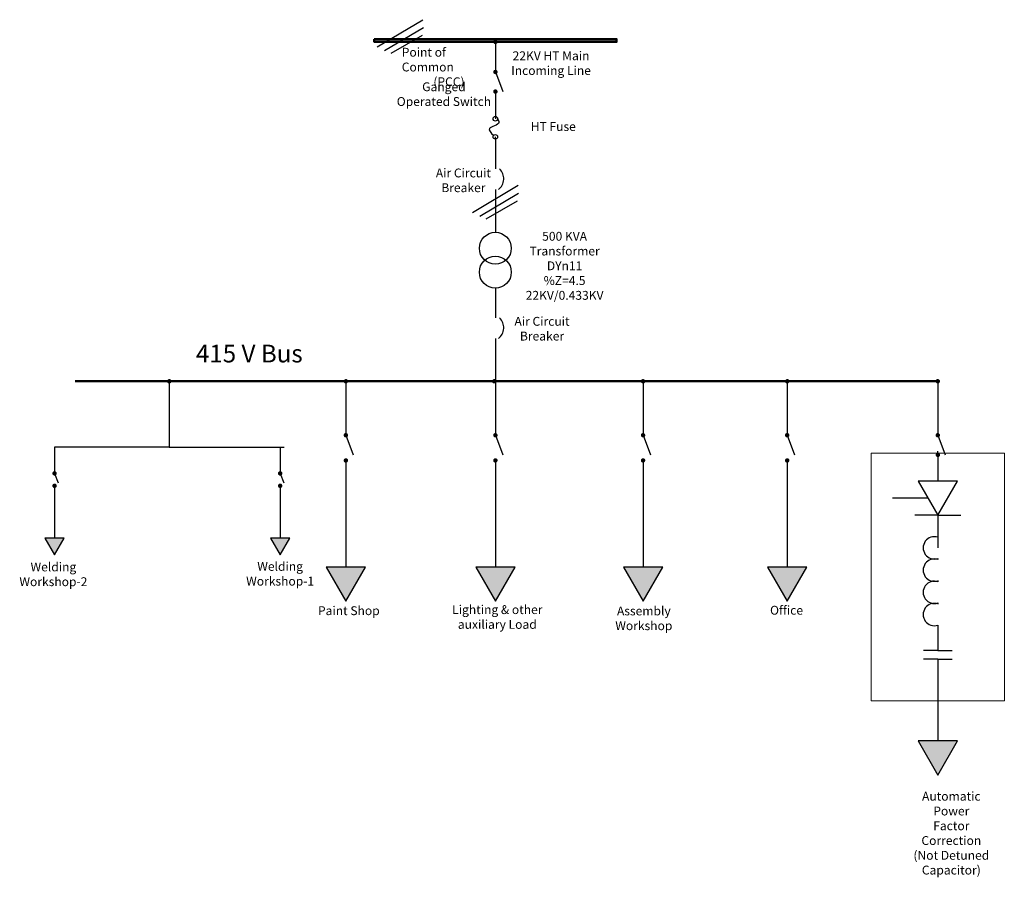
# Model space of a CAD drawing. Units: millimetres. Extents: x 147 to 258, y 68 to 165.
import ezdxf

# ---------------------------------------------------------------- set-up
doc = ezdxf.new("R2010")
doc.units = ezdxf.units.MM
doc.header["$MEASUREMENT"] = 0
for name, color, linetype, lineweight in [('E-ANNO-TEXT', 3, 'Continuous', 18), ('E-EQPM-BNDY', 8, 'Continuous', 18), ('E-POWR-BUSW', 1, 'Continuous', 50), ('E-POWR-WIRE', 7, 'Continuous', 25), ('E-SYMB', 4, 'Continuous', 25)]:
    doc.layers.add(name, color=color, linetype=linetype, lineweight=lineweight)
doc.styles.get("Standard").update_dxf_attribs({"font": 'arial.ttf'})

# ---------------------------------------------------------------- blocks, each defined once
blk = doc.blocks.new('LOAD-SYMBOL')
h = blk.add_hatch(color=256)
h.dxf.hatch_style = 1
h.paths.add_polyline_path([(202.61, 103), (198.16, 103), (200.38, 99.15)])
blk.add_lwpolyline([(200.38, 99.15), (202.61, 103), (198.16, 103)], close=True)
blk = doc.blocks.new('LOAD-SYMBOL-SMALL')
h = blk.add_hatch(color=256)
h.dxf.hatch_style = 1
h.paths.add_polyline_path([(150.59, 104.4), (151.68, 106.29), (149.5, 106.29)])
blk.add_lwpolyline([(150.59, 104.4), (151.68, 106.29), (149.5, 106.29)], close=True)
blk = doc.blocks.new('SWITCH-ISOLATOR')
blk.add_line((200.38, 117.9), (201.22, 115.7))
at = {"const_width": 0.25}
for points in [[(200.26, 117.9, 1), (200.51, 117.9, 1)], [(200.26, 115.05, 1), (200.51, 115.05, 1)]]:
    blk.add_lwpolyline(points, format="xyb", close=True, dxfattribs=at)
blk = doc.blocks.new('SWITCH-ISOLATOR-2')
blk.add_line((200.38, 158.91), (201.22, 156.7))
at = {"const_width": 0.25}
for points in [[(200.26, 158.91, 1), (200.51, 158.91, 1)], [(200.26, 156.7, 1), (200.51, 156.7, 1)]]:
    blk.add_lwpolyline(points, format="xyb", close=True, dxfattribs=at)
blk = doc.blocks.new('SWITCH-ISOLATOR-SMALL')
blk.add_line((150.59, 113.59), (151, 112.51))
at = {"const_width": 0.25}
for points in [[(150.47, 113.59, 1), (150.72, 113.59, 1)], [(150.47, 112.19, 1), (150.72, 112.19, 1)]]:
    blk.add_lwpolyline(points, format="xyb", close=True, dxfattribs=at)

msp = doc.modelspace()

# ---------------------------------------------------------------- hatches: boundary and pattern name
at = {"layer": 'E-POWR-BUSW'}
h = msp.add_hatch(color=256, dxfattribs=at)
h.dxf.hatch_style = 1
h.paths.add_polyline_path([(186.7, 162.31), (214.07, 162.31), (214.07, 162.63), (186.7, 162.63)])

# ---------------------------------------------------------------- linework, layer by layer
at = {"layer": 'E-EQPM-BNDY'}
msp.add_lwpolyline([(242.84, 115.89), (257.87, 115.89), (257.87, 87.9), (242.84, 87.9)], close=True, dxfattribs=at)
at = {"layer": 'E-POWR-BUSW'}
msp.add_line((152.94, 123.99), (250.36, 123.99), dxfattribs=at)
msp.add_lwpolyline([(186.7, 162.63), (214.07, 162.63), (214.07, 162.31), (186.7, 162.31)], close=True, dxfattribs=at)
at = {"layer": 'E-POWR-WIRE'}
for p, q in [((200.38, 162.31), (200.38, 158.91)), ((200.38, 156.7), (200.38, 153.89)), ((200.38, 153.89), (200.38, 153.63)), ((200.38, 151.33), (200.38, 151.59)), ((200.38, 151.33), (200.38, 147.98)), ((200.38, 145.64), (200.38, 140.81)), ((200.38, 134.51), (200.38, 131.15)), ((200.38, 128.81), (200.38, 123.99)), ((163.55, 123.99), (163.55, 116.57)), ((183.49, 123.99), (183.49, 117.9)), ((200.38, 123.99), (200.38, 117.9)), ((217.06, 123.99), (217.06, 117.9)), ((233.35, 123.99), (233.35, 117.9)), ((250.36, 123.99), (250.36, 117.9)), ((163.55, 116.57), (150.59, 116.57)), ((150.59, 116.57), (150.59, 113.59)), ((163.55, 116.57), (176.51, 116.57)), ((176.08, 116.57), (176.08, 113.59)), ((250.36, 115.68), (250.36, 116.1)), ((250.36, 115.68), (250.36, 112.72)), ((183.49, 115.05), (183.49, 112.24)), ((200.38, 115.05), (200.38, 112.24)), ((217.06, 115.05), (217.06, 112.24)), ((233.35, 115.05), (233.35, 112.24)), ((150.59, 112.19), (150.59, 110.81)), ((176.08, 112.19), (176.08, 110.81)), ((183.49, 112.24), (183.49, 103)), ((200.38, 112.24), (200.38, 103)), ((217.06, 112.24), (217.06, 103)), ((233.35, 112.24), (233.35, 103)), ((150.59, 110.81), (150.59, 106.29)), ((176.08, 110.81), (176.08, 106.29)), ((250.36, 108.86), (250.36, 105.18)), ((250.36, 103.99), (250.36, 103.86)), ((250.36, 101.48), (250.36, 101.35)), ((250.36, 98.97), (250.36, 98.84)), ((250.36, 96.46), (250.36, 93.6)), ((250.36, 92.62), (250.36, 83.38))]:
    msp.add_line(p, q, dxfattribs=at)
at = {"layer": 'E-SYMB'}
for p, q in [((187.04, 161.75), (192.19, 164.81)), ((187.87, 161.34), (192.26, 163.92)), ((188.6, 161.03), (192.14, 163.08)), ((197.79, 143.05), (202.94, 146.12)), ((198.62, 142.65), (203.01, 145.22)), ((199.35, 142.33), (202.89, 144.38)), ((249.24, 110.79), (245.22, 110.79)), ((250.36, 108.86), (247.76, 108.86)), ((250.36, 108.86), (252.95, 108.86)), ((250.36, 93.6), (248.73, 93.6)), ((250.36, 93.6), (251.98, 93.6)), ((250.36, 92.62), (248.73, 92.62)), ((250.36, 92.62), (251.98, 92.62))]:
    msp.add_line(p, q, dxfattribs=at)
at = {"layer": 'E-SYMB', "const_width": 0.25}
for points in [[(200.26, 162.31, 1), (200.51, 162.31, 1)], [(163.43, 123.99, 1), (163.68, 123.99, 1)], [(183.37, 123.99, 1), (183.62, 123.99, 1)], [(200.13, 123.99, 1), (200.38, 123.99, 1)], [(216.94, 123.99, 1), (217.19, 123.99, 1)], [(233.22, 123.99, 1), (233.47, 123.99, 1)], [(250.23, 123.99, 1), (250.48, 123.99, 1)]]:
    msp.add_lwpolyline(points, format="xyb", close=True, dxfattribs=at)
at = {"layer": 'E-SYMB'}
msp.add_lwpolyline([(250.36, 108.86), (252.58, 112.72), (248.13, 112.72)], close=True, dxfattribs=at)
for centre, radius in [((200.38, 153.63), 0.257), ((200.38, 151.59), 0.257), ((200.38, 139.01), 1.8), ((200.38, 136.31), 1.8)]:
    msp.add_circle(centre, radius, dxfattribs=at)
for centre, radius, start, end in [((199.79, 146.86), 1.54, 307.4337, 46.3448), ((199.79, 130.04), 1.54, 307.4337, 46.3448), ((249.96, 105.18), 1.26, 71.5267, 288.4733), ((249.96, 102.67), 1.26, 71.5267, 288.4733), ((249.96, 100.16), 1.26, 71.5267, 288.4733), ((249.96, 97.65), 1.26, 71.5267, 288.4733)]:
    msp.add_arc(centre, radius, start, end, dxfattribs=at)
msp.add_open_spline([(200.64, 153.63), (200.72, 153.49), (201.03, 152.91), (199.23, 152.7), (199.86, 152.05), (200.19, 151.76)], degree=3, knots=[0, 0, 0, 0, 0.432474, 1.710895, 2.673343, 2.673343, 2.673343, 2.673343], dxfattribs=at)

# ---------------------------------------------------------------- block references
for name, p in [('SWITCH-ISOLATOR-2', (0, 0)), ('SWITCH-ISOLATOR', (-16.89, 0)), ('SWITCH-ISOLATOR', (0, 0)), ('SWITCH-ISOLATOR', (16.68, 0)), ('SWITCH-ISOLATOR', (32.96, 0)), ('SWITCH-ISOLATOR-SMALL', (0, 0)), ('SWITCH-ISOLATOR-SMALL', (25.48, 0)), ('LOAD-SYMBOL-SMALL', (0, 0)), ('LOAD-SYMBOL-SMALL', (25.48, 0)), ('LOAD-SYMBOL', (-16.89, 0)), ('LOAD-SYMBOL', (0, 0)), ('LOAD-SYMBOL', (16.68, 0)), ('LOAD-SYMBOL', (32.96, 0)), ('LOAD-SYMBOL', (49.97, -19.62))]:
    msp.add_blockref(name, p, dxfattribs=at)
at = {"layer": 'E-SYMB', "rotation": 0.2273311619710558}
msp.add_blockref('SWITCH-ISOLATOR-2', (50.6, -41.81), dxfattribs=at)

# ---------------------------------------------------------------- texts
at = {"layer": 'E-ANNO-TEXT', "attachment_point": 1}
for s, width, insert, char_height in [('Point of Common\\P\\pxqc;(PCC)', 10.6637, (189.81, 161.64), 1), ('\\pxqc;22KV HT Main\\PIncoming Line', 10.6637, (201.34, 161.24), 1), ('\\pxqc;Ganged Operated Switch', 10.6637, (189.24, 157.74), 1), ('\\pxqc;HT Fuse', 10.6637, (201.59, 153.25), 1), ('\\pxqc;Air Circuit Breaker', 10.6637, (191.44, 148.01), 1), ('\\pxqc;500 KVA\\PTransformer\\PDYn11\\P%Z=4.5\\P22KV/0.433KV', 10.6637, (202.87, 140.86), 1), ('\\pxqc;Air Circuit Breaker', 10.6637, (200.32, 131.26), 1), ('415 V Bus', 15.9813, (166.56, 128.12), 2), ('\\pxqc;Welding\\PWorkshop-2', 10.6637, (145.13, 103.53), 1), ('\\pxqc;Welding\\PWorkshop-1', 10.6637, (170.74, 103.59), 1), ('\\pxqc;Paint Shop', 10.6637, (178.5, 98.59), 1), ('\\pxqc;Lighting & other\\Pauxiliary Load', 10.6637, (195.27, 98.71), 1), ('\\pxqc;Assembly\\PWorkshop', 10.6637, (211.82, 98.56), 1), ('\\pxqc;Office', 10.6637, (227.94, 98.64), 1), ('\\pxqc;Automatic Power\\PFactor Correction\\P(Not Detuned\\PCapacitor)', 10.6637, (246.55, 77.64), 1)]:
    msp.add_mtext_dynamic_manual_height_columns(s, width=width, gutter_width=1, heights=[0], dxfattribs=dict(at, insert=insert, char_height=char_height))

doc.saveas('drawing.dxf')
